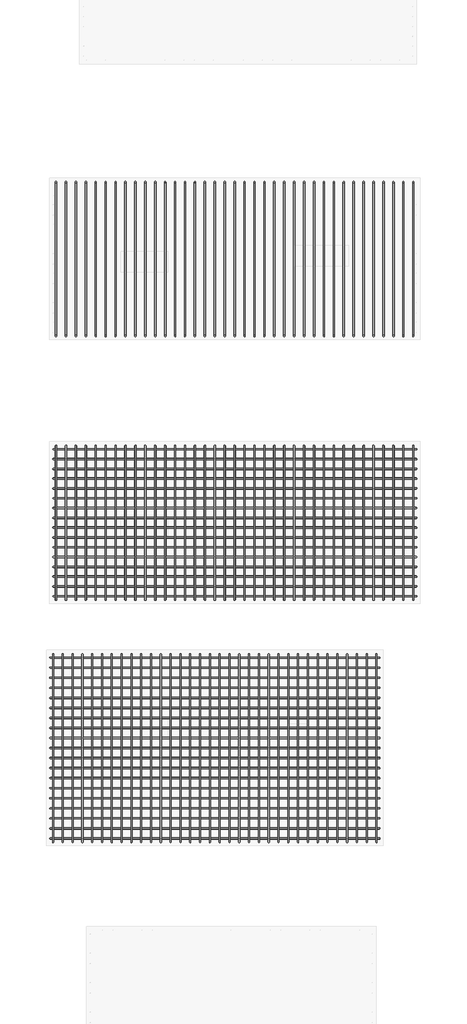
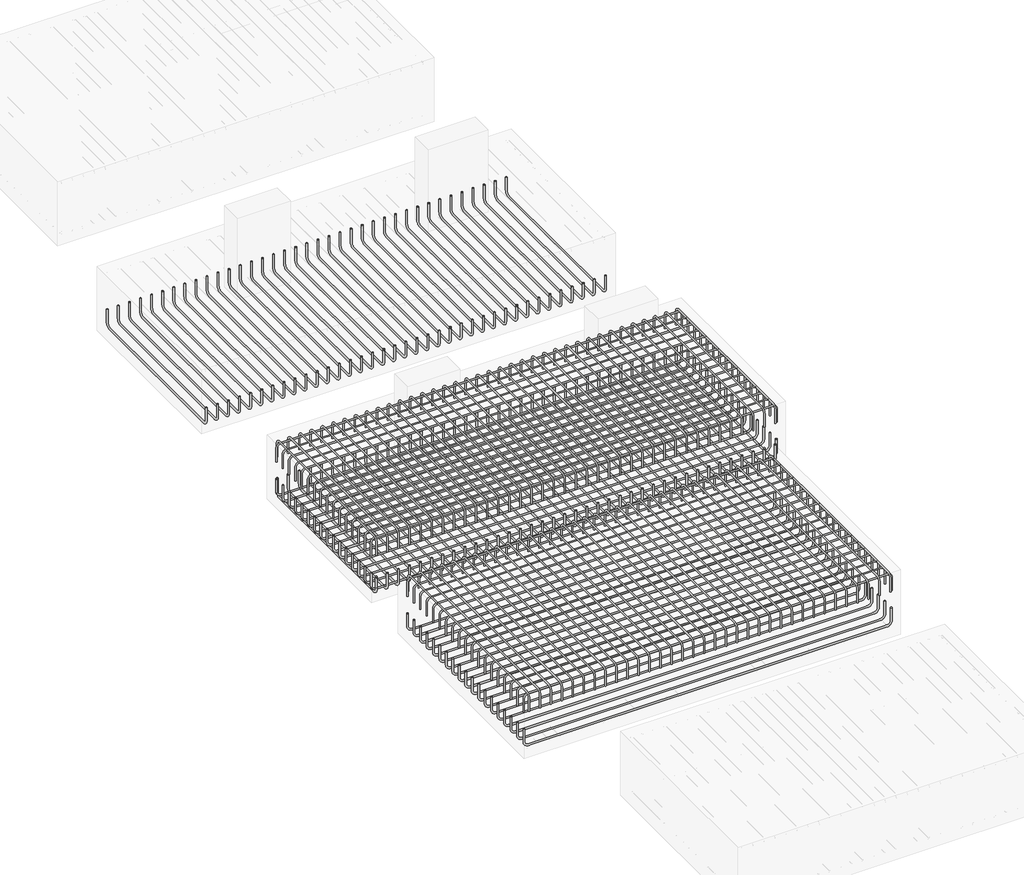
# One storey, part 7 of 21: 8 reinforcing bars.
"""IFC4 building model written with IfcOpenShell, lengths in millimetres."""

from ifc_helpers import new_model, si_unit, point, frame, origin, place, context, project, spatial, polyline, circle_curve, trimmed, segment, composite_curve, source, transform, mapped, element, save
from ifc_brep_helpers import swept_disk

model = new_model("IFC4")

# Units and contexts
model_context = context("Model", 3, world=origin())
ifc_project = project(units=[si_unit("LENGTHUNIT", "METRE", prefix="MILLI")], contexts=[model_context])

# Site, building, storey
site = spatial("IfcSite", under=ifc_project)
building = spatial("IfcBuilding", under=site)
storey = spatial("IfcBuildingStorey", under=building, Elevation=-1100.0)

# Reinforcing bars
placement = place(None, origin())
reinforcing_bar_shape = source(origin(), model_context, "Body", "SolidModel", [
    swept_disk(composite_curve([segment(polyline([(10485.4160849, 639.1704288, -1700.0), (10485.4160849, 639.1704288, -1882.5)]), True, "CONTINUOUS"), segment(trimmed(circle_curve(frame((10485.4160849, 581.6704288, -1882.5), z_axis=(-1.0, 0.0, 0.0), x_axis=(0.0, 57.5, 0.0)), 57.5), [point((10485.4160849, 639.1704288, -1882.5))], [point((10485.4160849, 581.6704288, -1940.0))], True, "CARTESIAN"), True, "CONTINUOUS"), segment(polyline([(10485.4160849, 581.6704288, -1940.0), (10485.4160849, -1583.3295712, -1940.0)]), True, "CONTINUOUS"), segment(trimmed(circle_curve(frame((10485.4160849, -1583.3295712, -1882.5), z_axis=(-1.0, 0.0, 0.0), x_axis=(0.0, 0.0, -57.5)), 57.5), [point((10485.4160849, -1583.3295712, -1940.0))], [point((10485.4160849, -1640.8295712, -1882.5))], True, "CARTESIAN"), True, "CONTINUOUS"), segment(polyline([(10485.4160849, -1640.8295712, -1882.5), (10485.4160849, -1640.8295712, -1700.0)]), True, "CONTINUOUS")], self_intersect=False), 10.0),
])
element("IfcReinforcingBar", 1, at=placement, inside=storey, context=model_context, shape_type="MappedRepresentation", body=[
    mapped(reinforcing_bar_shape, transform((0.0, 0.0, 0.0), x_axis=(1.0, 0.0, 0.0), y_axis=(0.0, 1.0, 0.0), z_axis=(0.0, 0.0, 1.0))),
    mapped(reinforcing_bar_shape, transform((147.2696553, 0.0, 0.0), x_axis=(1.0, 0.0, 0.0), y_axis=(0.0, 1.0, 0.0), z_axis=(0.0, 0.0, 1.0))),
    mapped(reinforcing_bar_shape, transform((294.5393106, 0.0, 0.0), x_axis=(1.0, 0.0, 0.0), y_axis=(0.0, 1.0, 0.0), z_axis=(0.0, 0.0, 1.0))),
    mapped(reinforcing_bar_shape, transform((441.8089659, 0.0, 0.0), x_axis=(1.0, 0.0, 0.0), y_axis=(0.0, 1.0, 0.0), z_axis=(0.0, 0.0, 1.0))),
    mapped(reinforcing_bar_shape, transform((589.0786213, 0.0, 0.0), x_axis=(1.0, 0.0, 0.0), y_axis=(0.0, 1.0, 0.0), z_axis=(0.0, 0.0, 1.0))),
    mapped(reinforcing_bar_shape, transform((736.3482766, 0.0, 0.0), x_axis=(1.0, 0.0, 0.0), y_axis=(0.0, 1.0, 0.0), z_axis=(0.0, 0.0, 1.0))),
    mapped(reinforcing_bar_shape, transform((883.6179319, 0.0, 0.0), x_axis=(1.0, 0.0, 0.0), y_axis=(0.0, 1.0, 0.0), z_axis=(0.0, 0.0, 1.0))),
    mapped(reinforcing_bar_shape, transform((1030.8875872, 0.0, 0.0), x_axis=(1.0, 0.0, 0.0), y_axis=(0.0, 1.0, 0.0), z_axis=(0.0, 0.0, 1.0))),
    mapped(reinforcing_bar_shape, transform((1178.1572425, 0.0, 0.0), x_axis=(1.0, 0.0, 0.0), y_axis=(0.0, 1.0, 0.0), z_axis=(0.0, 0.0, 1.0))),
    mapped(reinforcing_bar_shape, transform((1325.4268978, 0.0, 0.0), x_axis=(1.0, 0.0, 0.0), y_axis=(0.0, 1.0, 0.0), z_axis=(0.0, 0.0, 1.0))),
    mapped(reinforcing_bar_shape, transform((1472.6965532, 0.0, 0.0), x_axis=(1.0, 0.0, 0.0), y_axis=(0.0, 1.0, 0.0), z_axis=(0.0, 0.0, 1.0))),
    mapped(reinforcing_bar_shape, transform((1619.9662085, 0.0, 0.0), x_axis=(1.0, 0.0, 0.0), y_axis=(0.0, 1.0, 0.0), z_axis=(0.0, 0.0, 1.0))),
    mapped(reinforcing_bar_shape, transform((1767.2358638, 0.0, 0.0), x_axis=(1.0, 0.0, 0.0), y_axis=(0.0, 1.0, 0.0), z_axis=(0.0, 0.0, 1.0))),
    mapped(reinforcing_bar_shape, transform((1914.5055191, 0.0, 0.0), x_axis=(1.0, 0.0, 0.0), y_axis=(0.0, 1.0, 0.0), z_axis=(0.0, 0.0, 1.0))),
    mapped(reinforcing_bar_shape, transform((2061.7751744, 0.0, 0.0), x_axis=(1.0, 0.0, 0.0), y_axis=(0.0, 1.0, 0.0), z_axis=(0.0, 0.0, 1.0))),
    mapped(reinforcing_bar_shape, transform((2209.0448297, 0.0, 0.0), x_axis=(1.0, 0.0, 0.0), y_axis=(0.0, 1.0, 0.0), z_axis=(0.0, 0.0, 1.0))),
    mapped(reinforcing_bar_shape, transform((2356.314485, 0.0, 0.0), x_axis=(1.0, 0.0, 0.0), y_axis=(0.0, 1.0, 0.0), z_axis=(0.0, 0.0, 1.0))),
    mapped(reinforcing_bar_shape, transform((2503.5841404, 0.0, 0.0), x_axis=(1.0, 0.0, 0.0), y_axis=(0.0, 1.0, 0.0), z_axis=(0.0, 0.0, 1.0))),
    mapped(reinforcing_bar_shape, transform((2650.8537957, 0.0, 0.0), x_axis=(1.0, 0.0, 0.0), y_axis=(0.0, 1.0, 0.0), z_axis=(0.0, 0.0, 1.0))),
    mapped(reinforcing_bar_shape, transform((2798.123451, 0.0, 0.0), x_axis=(1.0, 0.0, 0.0), y_axis=(0.0, 1.0, 0.0), z_axis=(0.0, 0.0, 1.0))),
    mapped(reinforcing_bar_shape, transform((2945.3931063, 0.0, 0.0), x_axis=(1.0, 0.0, 0.0), y_axis=(0.0, 1.0, 0.0), z_axis=(0.0, 0.0, 1.0))),
    mapped(reinforcing_bar_shape, transform((3092.6627616, 0.0, 0.0), x_axis=(1.0, 0.0, 0.0), y_axis=(0.0, 1.0, 0.0), z_axis=(0.0, 0.0, 1.0))),
    mapped(reinforcing_bar_shape, transform((3239.9324169, 0.0, 0.0), x_axis=(1.0, 0.0, 0.0), y_axis=(0.0, 1.0, 0.0), z_axis=(0.0, 0.0, 1.0))),
    mapped(reinforcing_bar_shape, transform((3387.2020722, 0.0, 0.0), x_axis=(1.0, 0.0, 0.0), y_axis=(0.0, 1.0, 0.0), z_axis=(0.0, 0.0, 1.0))),
    mapped(reinforcing_bar_shape, transform((3534.4717276, 0.0, 0.0), x_axis=(1.0, 0.0, 0.0), y_axis=(0.0, 1.0, 0.0), z_axis=(0.0, 0.0, 1.0))),
    mapped(reinforcing_bar_shape, transform((3681.7413829, 0.0, 0.0), x_axis=(1.0, 0.0, 0.0), y_axis=(0.0, 1.0, 0.0), z_axis=(0.0, 0.0, 1.0))),
    mapped(reinforcing_bar_shape, transform((3829.0110382, 0.0, 0.0), x_axis=(1.0, 0.0, 0.0), y_axis=(0.0, 1.0, 0.0), z_axis=(0.0, 0.0, 1.0))),
    mapped(reinforcing_bar_shape, transform((3976.2806935, 0.0, 0.0), x_axis=(1.0, 0.0, 0.0), y_axis=(0.0, 1.0, 0.0), z_axis=(0.0, 0.0, 1.0))),
    mapped(reinforcing_bar_shape, transform((4123.5503488, 0.0, 0.0), x_axis=(1.0, 0.0, 0.0), y_axis=(0.0, 1.0, 0.0), z_axis=(0.0, 0.0, 1.0))),
    mapped(reinforcing_bar_shape, transform((4270.8200041, 0.0, 0.0), x_axis=(1.0, 0.0, 0.0), y_axis=(0.0, 1.0, 0.0), z_axis=(0.0, 0.0, 1.0))),
    mapped(reinforcing_bar_shape, transform((4418.0896595, 0.0, 0.0), x_axis=(1.0, 0.0, 0.0), y_axis=(0.0, 1.0, 0.0), z_axis=(0.0, 0.0, 1.0))),
    mapped(reinforcing_bar_shape, transform((4565.3593148, 0.0, 0.0), x_axis=(1.0, 0.0, 0.0), y_axis=(0.0, 1.0, 0.0), z_axis=(0.0, 0.0, 1.0))),
    mapped(reinforcing_bar_shape, transform((4712.6289701, 0.0, 0.0), x_axis=(1.0, 0.0, 0.0), y_axis=(0.0, 1.0, 0.0), z_axis=(0.0, 0.0, 1.0))),
    mapped(reinforcing_bar_shape, transform((4859.8986254, 0.0, 0.0), x_axis=(1.0, 0.0, 0.0), y_axis=(0.0, 1.0, 0.0), z_axis=(0.0, 0.0, 1.0))),
    mapped(reinforcing_bar_shape, transform((5007.1682807, 0.0, 0.0), x_axis=(1.0, 0.0, 0.0), y_axis=(0.0, 1.0, 0.0), z_axis=(0.0, 0.0, 1.0))),
    mapped(reinforcing_bar_shape, transform((5154.437936, 0.0, 0.0), x_axis=(1.0, 0.0, 0.0), y_axis=(0.0, 1.0, 0.0), z_axis=(0.0, 0.0, 1.0))),
    mapped(reinforcing_bar_shape, transform((5301.7075913, 0.0, 0.0), x_axis=(1.0, 0.0, 0.0), y_axis=(0.0, 1.0, 0.0), z_axis=(0.0, 0.0, 1.0))),
])
reinforcing_bar_2_shape = source(origin(), model_context, "Body", "SolidModel", [
    swept_disk(composite_curve([segment(polyline([(10485.4160849, -3270.8295712, -1700.0), (10485.4160849, -3270.8295712, -1882.5)]), True, "CONTINUOUS"), segment(trimmed(circle_curve(frame((10485.4160849, -3328.3295712, -1882.5), z_axis=(-1.0, 0.0, 0.0), x_axis=(0.0, 57.5, 0.0)), 57.5), [point((10485.4160849, -3270.8295712, -1882.5))], [point((10485.4160849, -3328.3295712, -1940.0))], True, "CARTESIAN"), True, "CONTINUOUS"), segment(polyline([(10485.4160849, -3328.3295712, -1940.0), (10485.4160849, -5493.3295712, -1940.0)]), True, "CONTINUOUS"), segment(trimmed(circle_curve(frame((10485.4160849, -5493.3295712, -1882.5), z_axis=(-1.0, 0.0, 0.0), x_axis=(0.0, 0.0, -57.5)), 57.5), [point((10485.4160849, -5493.3295712, -1940.0))], [point((10485.4160849, -5550.8295712, -1882.5))], True, "CARTESIAN"), True, "CONTINUOUS"), segment(polyline([(10485.4160849, -5550.8295712, -1882.5), (10485.4160849, -5550.8295712, -1700.0)]), True, "CONTINUOUS")], self_intersect=False), 10.0),
])
element("IfcReinforcingBar", 2, at=placement, inside=storey, context=model_context, shape_type="MappedRepresentation", body=[
    mapped(reinforcing_bar_2_shape, transform((0.0, 0.0, 0.0), x_axis=(1.0, 0.0, 0.0), y_axis=(0.0, 1.0, 0.0), z_axis=(0.0, 0.0, 1.0))),
    mapped(reinforcing_bar_2_shape, transform((147.2696553, 0.0, 0.0), x_axis=(1.0, 0.0, 0.0), y_axis=(0.0, 1.0, 0.0), z_axis=(0.0, 0.0, 1.0))),
    mapped(reinforcing_bar_2_shape, transform((294.5393106, 0.0, 0.0), x_axis=(1.0, 0.0, 0.0), y_axis=(0.0, 1.0, 0.0), z_axis=(0.0, 0.0, 1.0))),
    mapped(reinforcing_bar_2_shape, transform((441.8089659, 0.0, 0.0), x_axis=(1.0, 0.0, 0.0), y_axis=(0.0, 1.0, 0.0), z_axis=(0.0, 0.0, 1.0))),
    mapped(reinforcing_bar_2_shape, transform((589.0786213, 0.0, 0.0), x_axis=(1.0, 0.0, 0.0), y_axis=(0.0, 1.0, 0.0), z_axis=(0.0, 0.0, 1.0))),
    mapped(reinforcing_bar_2_shape, transform((736.3482766, 0.0, 0.0), x_axis=(1.0, 0.0, 0.0), y_axis=(0.0, 1.0, 0.0), z_axis=(0.0, 0.0, 1.0))),
    mapped(reinforcing_bar_2_shape, transform((883.6179319, 0.0, 0.0), x_axis=(1.0, 0.0, 0.0), y_axis=(0.0, 1.0, 0.0), z_axis=(0.0, 0.0, 1.0))),
    mapped(reinforcing_bar_2_shape, transform((1030.8875872, 0.0, 0.0), x_axis=(1.0, 0.0, 0.0), y_axis=(0.0, 1.0, 0.0), z_axis=(0.0, 0.0, 1.0))),
    mapped(reinforcing_bar_2_shape, transform((1178.1572425, 0.0, 0.0), x_axis=(1.0, 0.0, 0.0), y_axis=(0.0, 1.0, 0.0), z_axis=(0.0, 0.0, 1.0))),
    mapped(reinforcing_bar_2_shape, transform((1325.4268978, 0.0, 0.0), x_axis=(1.0, 0.0, 0.0), y_axis=(0.0, 1.0, 0.0), z_axis=(0.0, 0.0, 1.0))),
    mapped(reinforcing_bar_2_shape, transform((1472.6965532, 0.0, 0.0), x_axis=(1.0, 0.0, 0.0), y_axis=(0.0, 1.0, 0.0), z_axis=(0.0, 0.0, 1.0))),
    mapped(reinforcing_bar_2_shape, transform((1619.9662085, 0.0, 0.0), x_axis=(1.0, 0.0, 0.0), y_axis=(0.0, 1.0, 0.0), z_axis=(0.0, 0.0, 1.0))),
    mapped(reinforcing_bar_2_shape, transform((1767.2358638, 0.0, 0.0), x_axis=(1.0, 0.0, 0.0), y_axis=(0.0, 1.0, 0.0), z_axis=(0.0, 0.0, 1.0))),
    mapped(reinforcing_bar_2_shape, transform((1914.5055191, 0.0, 0.0), x_axis=(1.0, 0.0, 0.0), y_axis=(0.0, 1.0, 0.0), z_axis=(0.0, 0.0, 1.0))),
    mapped(reinforcing_bar_2_shape, transform((2061.7751744, 0.0, 0.0), x_axis=(1.0, 0.0, 0.0), y_axis=(0.0, 1.0, 0.0), z_axis=(0.0, 0.0, 1.0))),
    mapped(reinforcing_bar_2_shape, transform((2209.0448297, 0.0, 0.0), x_axis=(1.0, 0.0, 0.0), y_axis=(0.0, 1.0, 0.0), z_axis=(0.0, 0.0, 1.0))),
    mapped(reinforcing_bar_2_shape, transform((2356.314485, 0.0, 0.0), x_axis=(1.0, 0.0, 0.0), y_axis=(0.0, 1.0, 0.0), z_axis=(0.0, 0.0, 1.0))),
    mapped(reinforcing_bar_2_shape, transform((2503.5841404, 0.0, 0.0), x_axis=(1.0, 0.0, 0.0), y_axis=(0.0, 1.0, 0.0), z_axis=(0.0, 0.0, 1.0))),
    mapped(reinforcing_bar_2_shape, transform((2650.8537957, 0.0, 0.0), x_axis=(1.0, 0.0, 0.0), y_axis=(0.0, 1.0, 0.0), z_axis=(0.0, 0.0, 1.0))),
    mapped(reinforcing_bar_2_shape, transform((2798.123451, 0.0, 0.0), x_axis=(1.0, 0.0, 0.0), y_axis=(0.0, 1.0, 0.0), z_axis=(0.0, 0.0, 1.0))),
    mapped(reinforcing_bar_2_shape, transform((2945.3931063, 0.0, 0.0), x_axis=(1.0, 0.0, 0.0), y_axis=(0.0, 1.0, 0.0), z_axis=(0.0, 0.0, 1.0))),
    mapped(reinforcing_bar_2_shape, transform((3092.6627616, 0.0, 0.0), x_axis=(1.0, 0.0, 0.0), y_axis=(0.0, 1.0, 0.0), z_axis=(0.0, 0.0, 1.0))),
    mapped(reinforcing_bar_2_shape, transform((3239.9324169, 0.0, 0.0), x_axis=(1.0, 0.0, 0.0), y_axis=(0.0, 1.0, 0.0), z_axis=(0.0, 0.0, 1.0))),
    mapped(reinforcing_bar_2_shape, transform((3387.2020722, 0.0, 0.0), x_axis=(1.0, 0.0, 0.0), y_axis=(0.0, 1.0, 0.0), z_axis=(0.0, 0.0, 1.0))),
    mapped(reinforcing_bar_2_shape, transform((3534.4717276, 0.0, 0.0), x_axis=(1.0, 0.0, 0.0), y_axis=(0.0, 1.0, 0.0), z_axis=(0.0, 0.0, 1.0))),
    mapped(reinforcing_bar_2_shape, transform((3681.7413829, 0.0, 0.0), x_axis=(1.0, 0.0, 0.0), y_axis=(0.0, 1.0, 0.0), z_axis=(0.0, 0.0, 1.0))),
    mapped(reinforcing_bar_2_shape, transform((3829.0110382, 0.0, 0.0), x_axis=(1.0, 0.0, 0.0), y_axis=(0.0, 1.0, 0.0), z_axis=(0.0, 0.0, 1.0))),
    mapped(reinforcing_bar_2_shape, transform((3976.2806935, 0.0, 0.0), x_axis=(1.0, 0.0, 0.0), y_axis=(0.0, 1.0, 0.0), z_axis=(0.0, 0.0, 1.0))),
    mapped(reinforcing_bar_2_shape, transform((4123.5503488, 0.0, 0.0), x_axis=(1.0, 0.0, 0.0), y_axis=(0.0, 1.0, 0.0), z_axis=(0.0, 0.0, 1.0))),
    mapped(reinforcing_bar_2_shape, transform((4270.8200041, 0.0, 0.0), x_axis=(1.0, 0.0, 0.0), y_axis=(0.0, 1.0, 0.0), z_axis=(0.0, 0.0, 1.0))),
    mapped(reinforcing_bar_2_shape, transform((4418.0896595, 0.0, 0.0), x_axis=(1.0, 0.0, 0.0), y_axis=(0.0, 1.0, 0.0), z_axis=(0.0, 0.0, 1.0))),
    mapped(reinforcing_bar_2_shape, transform((4565.3593148, 0.0, 0.0), x_axis=(1.0, 0.0, 0.0), y_axis=(0.0, 1.0, 0.0), z_axis=(0.0, 0.0, 1.0))),
    mapped(reinforcing_bar_2_shape, transform((4712.6289701, 0.0, 0.0), x_axis=(1.0, 0.0, 0.0), y_axis=(0.0, 1.0, 0.0), z_axis=(0.0, 0.0, 1.0))),
    mapped(reinforcing_bar_2_shape, transform((4859.8986254, 0.0, 0.0), x_axis=(1.0, 0.0, 0.0), y_axis=(0.0, 1.0, 0.0), z_axis=(0.0, 0.0, 1.0))),
    mapped(reinforcing_bar_2_shape, transform((5007.1682807, 0.0, 0.0), x_axis=(1.0, 0.0, 0.0), y_axis=(0.0, 1.0, 0.0), z_axis=(0.0, 0.0, 1.0))),
    mapped(reinforcing_bar_2_shape, transform((5154.437936, 0.0, 0.0), x_axis=(1.0, 0.0, 0.0), y_axis=(0.0, 1.0, 0.0), z_axis=(0.0, 0.0, 1.0))),
    mapped(reinforcing_bar_2_shape, transform((5301.7075913, 0.0, 0.0), x_axis=(1.0, 0.0, 0.0), y_axis=(0.0, 1.0, 0.0), z_axis=(0.0, 0.0, 1.0))),
])
reinforcing_bar_3_shape = source(origin(), model_context, "Body", "SolidModel", [
    swept_disk(composite_curve([segment(polyline([(10485.4160849, -5552.8795712, -1400.0), (10485.4160849, -5552.8795712, -1213.4)]), True, "CONTINUOUS"), segment(trimmed(circle_curve(frame((10485.4160849, -5497.4295712, -1213.4), z_axis=(-1.0, 0.0, 0.0), x_axis=(0.0, -55.44999999999982, 0.0)), 55.45), [point((10485.4160849, -5552.8795712, -1213.4))], [point((10485.4160849, -5497.4295712, -1157.95))], True, "CARTESIAN"), True, "CONTINUOUS"), segment(polyline([(10485.4160849, -5497.4295712, -1157.95), (10485.4160849, -3324.2295712, -1157.95)]), True, "CONTINUOUS"), segment(trimmed(circle_curve(frame((10485.4160849, -3324.2295712, -1213.4), z_axis=(-1.0, 0.0, 0.0), x_axis=(0.0, 0.0, 55.450000000000045)), 55.45), [point((10485.4160849, -3324.2295712, -1157.95))], [point((10485.4160849, -3268.7795712, -1213.4))], True, "CARTESIAN"), True, "CONTINUOUS"), segment(polyline([(10485.4160849, -3268.7795712, -1213.4), (10485.4160849, -3268.7795712, -1400.0)]), True, "CONTINUOUS")], self_intersect=False), 7.95),
])
element("IfcReinforcingBar", 3, at=placement, inside=storey, context=model_context, shape_type="MappedRepresentation", body=[
    mapped(reinforcing_bar_3_shape, transform((0.0, 0.0, 0.0), x_axis=(1.0, 0.0, 0.0), y_axis=(0.0, 1.0, 0.0), z_axis=(0.0, 0.0, 1.0))),
    mapped(reinforcing_bar_3_shape, transform((147.2696553, 0.0, 0.0), x_axis=(1.0, 0.0, 0.0), y_axis=(0.0, 1.0, 0.0), z_axis=(0.0, 0.0, 1.0))),
    mapped(reinforcing_bar_3_shape, transform((294.5393106, 0.0, 0.0), x_axis=(1.0, 0.0, 0.0), y_axis=(0.0, 1.0, 0.0), z_axis=(0.0, 0.0, 1.0))),
    mapped(reinforcing_bar_3_shape, transform((441.8089659, 0.0, 0.0), x_axis=(1.0, 0.0, 0.0), y_axis=(0.0, 1.0, 0.0), z_axis=(0.0, 0.0, 1.0))),
    mapped(reinforcing_bar_3_shape, transform((589.0786213, 0.0, 0.0), x_axis=(1.0, 0.0, 0.0), y_axis=(0.0, 1.0, 0.0), z_axis=(0.0, 0.0, 1.0))),
    mapped(reinforcing_bar_3_shape, transform((736.3482766, 0.0, 0.0), x_axis=(1.0, 0.0, 0.0), y_axis=(0.0, 1.0, 0.0), z_axis=(0.0, 0.0, 1.0))),
    mapped(reinforcing_bar_3_shape, transform((883.6179319, 0.0, 0.0), x_axis=(1.0, 0.0, 0.0), y_axis=(0.0, 1.0, 0.0), z_axis=(0.0, 0.0, 1.0))),
    mapped(reinforcing_bar_3_shape, transform((1030.8875872, 0.0, 0.0), x_axis=(1.0, 0.0, 0.0), y_axis=(0.0, 1.0, 0.0), z_axis=(0.0, 0.0, 1.0))),
    mapped(reinforcing_bar_3_shape, transform((1178.1572425, 0.0, 0.0), x_axis=(1.0, 0.0, 0.0), y_axis=(0.0, 1.0, 0.0), z_axis=(0.0, 0.0, 1.0))),
    mapped(reinforcing_bar_3_shape, transform((1325.4268978, 0.0, 0.0), x_axis=(1.0, 0.0, 0.0), y_axis=(0.0, 1.0, 0.0), z_axis=(0.0, 0.0, 1.0))),
    mapped(reinforcing_bar_3_shape, transform((1472.6965532, 0.0, 0.0), x_axis=(1.0, 0.0, 0.0), y_axis=(0.0, 1.0, 0.0), z_axis=(0.0, 0.0, 1.0))),
    mapped(reinforcing_bar_3_shape, transform((1619.9662085, 0.0, 0.0), x_axis=(1.0, 0.0, 0.0), y_axis=(0.0, 1.0, 0.0), z_axis=(0.0, 0.0, 1.0))),
    mapped(reinforcing_bar_3_shape, transform((1767.2358638, 0.0, 0.0), x_axis=(1.0, 0.0, 0.0), y_axis=(0.0, 1.0, 0.0), z_axis=(0.0, 0.0, 1.0))),
    mapped(reinforcing_bar_3_shape, transform((1914.5055191, 0.0, 0.0), x_axis=(1.0, 0.0, 0.0), y_axis=(0.0, 1.0, 0.0), z_axis=(0.0, 0.0, 1.0))),
    mapped(reinforcing_bar_3_shape, transform((2061.7751744, 0.0, 0.0), x_axis=(1.0, 0.0, 0.0), y_axis=(0.0, 1.0, 0.0), z_axis=(0.0, 0.0, 1.0))),
    mapped(reinforcing_bar_3_shape, transform((2209.0448297, 0.0, 0.0), x_axis=(1.0, 0.0, 0.0), y_axis=(0.0, 1.0, 0.0), z_axis=(0.0, 0.0, 1.0))),
    mapped(reinforcing_bar_3_shape, transform((2356.314485, 0.0, 0.0), x_axis=(1.0, 0.0, 0.0), y_axis=(0.0, 1.0, 0.0), z_axis=(0.0, 0.0, 1.0))),
    mapped(reinforcing_bar_3_shape, transform((2503.5841404, 0.0, 0.0), x_axis=(1.0, 0.0, 0.0), y_axis=(0.0, 1.0, 0.0), z_axis=(0.0, 0.0, 1.0))),
    mapped(reinforcing_bar_3_shape, transform((2650.8537957, 0.0, 0.0), x_axis=(1.0, 0.0, 0.0), y_axis=(0.0, 1.0, 0.0), z_axis=(0.0, 0.0, 1.0))),
    mapped(reinforcing_bar_3_shape, transform((2798.123451, 0.0, 0.0), x_axis=(1.0, 0.0, 0.0), y_axis=(0.0, 1.0, 0.0), z_axis=(0.0, 0.0, 1.0))),
    mapped(reinforcing_bar_3_shape, transform((2945.3931063, 0.0, 0.0), x_axis=(1.0, 0.0, 0.0), y_axis=(0.0, 1.0, 0.0), z_axis=(0.0, 0.0, 1.0))),
    mapped(reinforcing_bar_3_shape, transform((3092.6627616, 0.0, 0.0), x_axis=(1.0, 0.0, 0.0), y_axis=(0.0, 1.0, 0.0), z_axis=(0.0, 0.0, 1.0))),
    mapped(reinforcing_bar_3_shape, transform((3239.9324169, 0.0, 0.0), x_axis=(1.0, 0.0, 0.0), y_axis=(0.0, 1.0, 0.0), z_axis=(0.0, 0.0, 1.0))),
    mapped(reinforcing_bar_3_shape, transform((3387.2020722, 0.0, 0.0), x_axis=(1.0, 0.0, 0.0), y_axis=(0.0, 1.0, 0.0), z_axis=(0.0, 0.0, 1.0))),
    mapped(reinforcing_bar_3_shape, transform((3534.4717276, 0.0, 0.0), x_axis=(1.0, 0.0, 0.0), y_axis=(0.0, 1.0, 0.0), z_axis=(0.0, 0.0, 1.0))),
    mapped(reinforcing_bar_3_shape, transform((3681.7413829, 0.0, 0.0), x_axis=(1.0, 0.0, 0.0), y_axis=(0.0, 1.0, 0.0), z_axis=(0.0, 0.0, 1.0))),
    mapped(reinforcing_bar_3_shape, transform((3829.0110382, 0.0, 0.0), x_axis=(1.0, 0.0, 0.0), y_axis=(0.0, 1.0, 0.0), z_axis=(0.0, 0.0, 1.0))),
    mapped(reinforcing_bar_3_shape, transform((3976.2806935, 0.0, 0.0), x_axis=(1.0, 0.0, 0.0), y_axis=(0.0, 1.0, 0.0), z_axis=(0.0, 0.0, 1.0))),
    mapped(reinforcing_bar_3_shape, transform((4123.5503488, 0.0, 0.0), x_axis=(1.0, 0.0, 0.0), y_axis=(0.0, 1.0, 0.0), z_axis=(0.0, 0.0, 1.0))),
    mapped(reinforcing_bar_3_shape, transform((4270.8200041, 0.0, 0.0), x_axis=(1.0, 0.0, 0.0), y_axis=(0.0, 1.0, 0.0), z_axis=(0.0, 0.0, 1.0))),
    mapped(reinforcing_bar_3_shape, transform((4418.0896595, 0.0, 0.0), x_axis=(1.0, 0.0, 0.0), y_axis=(0.0, 1.0, 0.0), z_axis=(0.0, 0.0, 1.0))),
    mapped(reinforcing_bar_3_shape, transform((4565.3593148, 0.0, 0.0), x_axis=(1.0, 0.0, 0.0), y_axis=(0.0, 1.0, 0.0), z_axis=(0.0, 0.0, 1.0))),
    mapped(reinforcing_bar_3_shape, transform((4712.6289701, 0.0, 0.0), x_axis=(1.0, 0.0, 0.0), y_axis=(0.0, 1.0, 0.0), z_axis=(0.0, 0.0, 1.0))),
    mapped(reinforcing_bar_3_shape, transform((4859.8986254, 0.0, 0.0), x_axis=(1.0, 0.0, 0.0), y_axis=(0.0, 1.0, 0.0), z_axis=(0.0, 0.0, 1.0))),
    mapped(reinforcing_bar_3_shape, transform((5007.1682807, 0.0, 0.0), x_axis=(1.0, 0.0, 0.0), y_axis=(0.0, 1.0, 0.0), z_axis=(0.0, 0.0, 1.0))),
    mapped(reinforcing_bar_3_shape, transform((5154.437936, 0.0, 0.0), x_axis=(1.0, 0.0, 0.0), y_axis=(0.0, 1.0, 0.0), z_axis=(0.0, 0.0, 1.0))),
    mapped(reinforcing_bar_3_shape, transform((5301.7075913, 0.0, 0.0), x_axis=(1.0, 0.0, 0.0), y_axis=(0.0, 1.0, 0.0), z_axis=(0.0, 0.0, 1.0))),
])
reinforcing_bar_4_shape = source(origin(), model_context, "Body", "SolidModel", [
    swept_disk(composite_curve([segment(polyline([(10447.1173137, -3320.6137352, -1428.1111113), (10447.1173137, -3320.6137352, -1241.5111113)]), True, "CONTINUOUS"), segment(trimmed(circle_curve(frame((10502.5673137, -3320.6137352, -1241.5111113), z_axis=(0.0, 1.0, 0.0), x_axis=(-55.44999999999891, 0.0, 0.0)), 55.45), [point((10447.1173137, -3320.6137352, -1241.5111113))], [point((10502.5673137, -3320.6137352, -1186.0611113))], True, "CARTESIAN"), True, "CONTINUOUS"), segment(polyline([(10502.5673137, -3320.6137352, -1186.0611113), (15775.7673137, -3320.6137352, -1186.0611113)]), True, "CONTINUOUS"), segment(trimmed(circle_curve(frame((15775.7673137, -3320.6137352, -1241.5111113), z_axis=(0.0, 1.0, 0.0), x_axis=(0.0, 0.0, 55.450000000000045)), 55.45), [point((15775.7673137, -3320.6137352, -1186.0611113))], [point((15831.2173137, -3320.6137352, -1241.5111113))], True, "CARTESIAN"), True, "CONTINUOUS"), segment(polyline([(15831.2173137, -3320.6137352, -1241.5111113), (15831.2173137, -3320.6137352, -1428.1111113)]), True, "CONTINUOUS")], self_intersect=False), 7.95),
])
element("IfcReinforcingBar", 4, at=placement, inside=storey, context=model_context, shape_type="MappedRepresentation", body=[
    mapped(reinforcing_bar_4_shape, transform((0.0, 0.0, 0.0), x_axis=(1.0, 0.0, 0.0), y_axis=(0.0, 1.0, 0.0), z_axis=(0.0, 0.0, 1.0))),
    mapped(reinforcing_bar_4_shape, transform((0.0, -145.2528929, 0.0), x_axis=(1.0, 0.0, 0.0), y_axis=(0.0, 1.0, 0.0), z_axis=(0.0, 0.0, 1.0))),
    mapped(reinforcing_bar_4_shape, transform((0.0, -290.5057858, 0.0), x_axis=(1.0, 0.0, 0.0), y_axis=(0.0, 1.0, 0.0), z_axis=(0.0, 0.0, 1.0))),
    mapped(reinforcing_bar_4_shape, transform((0.0, -435.7586787, 0.0), x_axis=(1.0, 0.0, 0.0), y_axis=(0.0, 1.0, 0.0), z_axis=(0.0, 0.0, 1.0))),
    mapped(reinforcing_bar_4_shape, transform((0.0, -581.0115716, 0.0), x_axis=(1.0, 0.0, 0.0), y_axis=(0.0, 1.0, 0.0), z_axis=(0.0, 0.0, 1.0))),
    mapped(reinforcing_bar_4_shape, transform((0.0, -726.2644645, 0.0), x_axis=(1.0, 0.0, 0.0), y_axis=(0.0, 1.0, 0.0), z_axis=(0.0, 0.0, 1.0))),
    mapped(reinforcing_bar_4_shape, transform((0.0, -871.5173574, 0.0), x_axis=(1.0, 0.0, 0.0), y_axis=(0.0, 1.0, 0.0), z_axis=(0.0, 0.0, 1.0))),
    mapped(reinforcing_bar_4_shape, transform((0.0, -1016.7702503, 0.0), x_axis=(1.0, 0.0, 0.0), y_axis=(0.0, 1.0, 0.0), z_axis=(0.0, 0.0, 1.0))),
    mapped(reinforcing_bar_4_shape, transform((0.0, -1162.0231432, 0.0), x_axis=(1.0, 0.0, 0.0), y_axis=(0.0, 1.0, 0.0), z_axis=(0.0, 0.0, 1.0))),
    mapped(reinforcing_bar_4_shape, transform((0.0, -1307.276036, 0.0), x_axis=(1.0, 0.0, 0.0), y_axis=(0.0, 1.0, 0.0), z_axis=(0.0, 0.0, 1.0))),
    mapped(reinforcing_bar_4_shape, transform((0.0, -1452.5289289, 0.0), x_axis=(1.0, 0.0, 0.0), y_axis=(0.0, 1.0, 0.0), z_axis=(0.0, 0.0, 1.0))),
    mapped(reinforcing_bar_4_shape, transform((0.0, -1597.7818218, 0.0), x_axis=(1.0, 0.0, 0.0), y_axis=(0.0, 1.0, 0.0), z_axis=(0.0, 0.0, 1.0))),
    mapped(reinforcing_bar_4_shape, transform((0.0, -1743.0347147, 0.0), x_axis=(1.0, 0.0, 0.0), y_axis=(0.0, 1.0, 0.0), z_axis=(0.0, 0.0, 1.0))),
    mapped(reinforcing_bar_4_shape, transform((0.0, -1888.2876076, 0.0), x_axis=(1.0, 0.0, 0.0), y_axis=(0.0, 1.0, 0.0), z_axis=(0.0, 0.0, 1.0))),
    mapped(reinforcing_bar_4_shape, transform((0.0, -2033.5405005, 0.0), x_axis=(1.0, 0.0, 0.0), y_axis=(0.0, 1.0, 0.0), z_axis=(0.0, 0.0, 1.0))),
    mapped(reinforcing_bar_4_shape, transform((0.0, -2178.7933934, 0.0), x_axis=(1.0, 0.0, 0.0), y_axis=(0.0, 1.0, 0.0), z_axis=(0.0, 0.0, 1.0))),
])
reinforcing_bar_5_shape = source(origin(), model_context, "Body", "SolidModel", [
    swept_disk(composite_curve([segment(polyline([(10449.1673137, -5499.4071286, -1669.8442859), (10449.1673137, -5499.4071286, -1852.3442859)]), True, "CONTINUOUS"), segment(trimmed(circle_curve(frame((10506.6673137, -5499.4071286, -1852.3442859), z_axis=(0.0, -1.0, 0.0), x_axis=(-57.5, 0.0, 0.0)), 57.5), [point((10449.1673137, -5499.4071286, -1852.3442859))], [point((10506.6673137, -5499.4071286, -1909.8442859))], True, "CARTESIAN"), True, "CONTINUOUS"), segment(polyline([(10506.6673137, -5499.4071286, -1909.8442859), (15771.6673137, -5499.4071286, -1909.8442859)]), True, "CONTINUOUS"), segment(trimmed(circle_curve(frame((15771.6673137, -5499.4071286, -1852.3442859), z_axis=(0.0, -1.0, 0.0), x_axis=(0.0, 0.0, -57.5)), 57.5), [point((15771.6673137, -5499.4071286, -1909.8442859))], [point((15829.1673137, -5499.4071286, -1852.3442859))], True, "CARTESIAN"), True, "CONTINUOUS"), segment(polyline([(15829.1673137, -5499.4071286, -1852.3442859), (15829.1673137, -5499.4071286, -1669.8442859)]), True, "CONTINUOUS")], self_intersect=False), 10.0),
])
element("IfcReinforcingBar", 5, at=placement, inside=storey, context=model_context, shape_type="MappedRepresentation", body=[
    mapped(reinforcing_bar_5_shape, transform((0.0, 0.0, 0.0), x_axis=(1.0, 0.0, 0.0), y_axis=(0.0, 1.0, 0.0), z_axis=(0.0, 0.0, 1.0))),
    mapped(reinforcing_bar_5_shape, transform((0.0, 145.2528929, 0.0), x_axis=(1.0, 0.0, 0.0), y_axis=(0.0, 1.0, 0.0), z_axis=(0.0, 0.0, 1.0))),
    mapped(reinforcing_bar_5_shape, transform((0.0, 290.5057858, 0.0), x_axis=(1.0, 0.0, 0.0), y_axis=(0.0, 1.0, 0.0), z_axis=(0.0, 0.0, 1.0))),
    mapped(reinforcing_bar_5_shape, transform((0.0, 435.7586787, 0.0), x_axis=(1.0, 0.0, 0.0), y_axis=(0.0, 1.0, 0.0), z_axis=(0.0, 0.0, 1.0))),
    mapped(reinforcing_bar_5_shape, transform((0.0, 581.0115716, 0.0), x_axis=(1.0, 0.0, 0.0), y_axis=(0.0, 1.0, 0.0), z_axis=(0.0, 0.0, 1.0))),
    mapped(reinforcing_bar_5_shape, transform((0.0, 726.2644645, 0.0), x_axis=(1.0, 0.0, 0.0), y_axis=(0.0, 1.0, 0.0), z_axis=(0.0, 0.0, 1.0))),
    mapped(reinforcing_bar_5_shape, transform((0.0, 871.5173574, 0.0), x_axis=(1.0, 0.0, 0.0), y_axis=(0.0, 1.0, 0.0), z_axis=(0.0, 0.0, 1.0))),
    mapped(reinforcing_bar_5_shape, transform((0.0, 1016.7702503, 0.0), x_axis=(1.0, 0.0, 0.0), y_axis=(0.0, 1.0, 0.0), z_axis=(0.0, 0.0, 1.0))),
    mapped(reinforcing_bar_5_shape, transform((0.0, 1162.0231432, 0.0), x_axis=(1.0, 0.0, 0.0), y_axis=(0.0, 1.0, 0.0), z_axis=(0.0, 0.0, 1.0))),
    mapped(reinforcing_bar_5_shape, transform((0.0, 1307.276036, 0.0), x_axis=(1.0, 0.0, 0.0), y_axis=(0.0, 1.0, 0.0), z_axis=(0.0, 0.0, 1.0))),
    mapped(reinforcing_bar_5_shape, transform((0.0, 1452.5289289, 0.0), x_axis=(1.0, 0.0, 0.0), y_axis=(0.0, 1.0, 0.0), z_axis=(0.0, 0.0, 1.0))),
    mapped(reinforcing_bar_5_shape, transform((0.0, 1597.7818218, 0.0), x_axis=(1.0, 0.0, 0.0), y_axis=(0.0, 1.0, 0.0), z_axis=(0.0, 0.0, 1.0))),
    mapped(reinforcing_bar_5_shape, transform((0.0, 1743.0347147, 0.0), x_axis=(1.0, 0.0, 0.0), y_axis=(0.0, 1.0, 0.0), z_axis=(0.0, 0.0, 1.0))),
    mapped(reinforcing_bar_5_shape, transform((0.0, 1888.2876076, 0.0), x_axis=(1.0, 0.0, 0.0), y_axis=(0.0, 1.0, 0.0), z_axis=(0.0, 0.0, 1.0))),
    mapped(reinforcing_bar_5_shape, transform((0.0, 2033.5405005, 0.0), x_axis=(1.0, 0.0, 0.0), y_axis=(0.0, 1.0, 0.0), z_axis=(0.0, 0.0, 1.0))),
    mapped(reinforcing_bar_5_shape, transform((0.0, 2178.7933934, 0.0), x_axis=(1.0, 0.0, 0.0), y_axis=(0.0, 1.0, 0.0), z_axis=(0.0, 0.0, 1.0))),
])
reinforcing_bar_6_shape = source(origin(), model_context, "Body", "SolidModel", [
    swept_disk(composite_curve([segment(polyline([(10440.4160849, -9142.8795712, -1400.0), (10440.4160849, -9142.8795712, -1213.4)]), True, "CONTINUOUS"), segment(trimmed(circle_curve(frame((10440.4160849, -9087.4295712, -1213.4), z_axis=(-1.0, 0.0, 0.0), x_axis=(0.0, -55.44999999999891, 0.0)), 55.45), [point((10440.4160849, -9142.8795712, -1213.4))], [point((10440.4160849, -9087.4295712, -1157.95))], True, "CARTESIAN"), True, "CONTINUOUS"), segment(polyline([(10440.4160849, -9087.4295712, -1157.95), (10440.4160849, -6414.2295712, -1157.95)]), True, "CONTINUOUS"), segment(trimmed(circle_curve(frame((10440.4160849, -6414.2295712, -1213.4), z_axis=(-1.0, 0.0, 0.0), x_axis=(0.0, 0.0, 55.450000000000045)), 55.45), [point((10440.4160849, -6414.2295712, -1157.95))], [point((10440.4160849, -6358.7795712, -1213.4))], True, "CARTESIAN"), True, "CONTINUOUS"), segment(polyline([(10440.4160849, -6358.7795712, -1213.4), (10440.4160849, -6358.7795712, -1400.0)]), True, "CONTINUOUS")], self_intersect=False), 7.95),
])
element("IfcReinforcingBar", 6, at=placement, inside=storey, context=model_context, shape_type="MappedRepresentation", body=[
    mapped(reinforcing_bar_6_shape, transform((0.0, 0.0, 0.0), x_axis=(1.0, 0.0, 0.0), y_axis=(0.0, 1.0, 0.0), z_axis=(0.0, 0.0, 1.0))),
    mapped(reinforcing_bar_6_shape, transform((145.5062906, 0.0, 0.0), x_axis=(1.0, 0.0, 0.0), y_axis=(0.0, 1.0, 0.0), z_axis=(0.0, 0.0, 1.0))),
    mapped(reinforcing_bar_6_shape, transform((291.0125813, 0.0, 0.0), x_axis=(1.0, 0.0, 0.0), y_axis=(0.0, 1.0, 0.0), z_axis=(0.0, 0.0, 1.0))),
    mapped(reinforcing_bar_6_shape, transform((436.5188719, 0.0, 0.0), x_axis=(1.0, 0.0, 0.0), y_axis=(0.0, 1.0, 0.0), z_axis=(0.0, 0.0, 1.0))),
    mapped(reinforcing_bar_6_shape, transform((582.0251626, 0.0, 0.0), x_axis=(1.0, 0.0, 0.0), y_axis=(0.0, 1.0, 0.0), z_axis=(0.0, 0.0, 1.0))),
    mapped(reinforcing_bar_6_shape, transform((727.5314532, 0.0, 0.0), x_axis=(1.0, 0.0, 0.0), y_axis=(0.0, 1.0, 0.0), z_axis=(0.0, 0.0, 1.0))),
    mapped(reinforcing_bar_6_shape, transform((873.0377439, 0.0, 0.0), x_axis=(1.0, 0.0, 0.0), y_axis=(0.0, 1.0, 0.0), z_axis=(0.0, 0.0, 1.0))),
    mapped(reinforcing_bar_6_shape, transform((1018.5440345, 0.0, 0.0), x_axis=(1.0, 0.0, 0.0), y_axis=(0.0, 1.0, 0.0), z_axis=(0.0, 0.0, 1.0))),
    mapped(reinforcing_bar_6_shape, transform((1164.0503252, 0.0, 0.0), x_axis=(1.0, 0.0, 0.0), y_axis=(0.0, 1.0, 0.0), z_axis=(0.0, 0.0, 1.0))),
    mapped(reinforcing_bar_6_shape, transform((1309.5566158, 0.0, 0.0), x_axis=(1.0, 0.0, 0.0), y_axis=(0.0, 1.0, 0.0), z_axis=(0.0, 0.0, 1.0))),
    mapped(reinforcing_bar_6_shape, transform((1455.0629065, 0.0, 0.0), x_axis=(1.0, 0.0, 0.0), y_axis=(0.0, 1.0, 0.0), z_axis=(0.0, 0.0, 1.0))),
    mapped(reinforcing_bar_6_shape, transform((1600.5691971, 0.0, 0.0), x_axis=(1.0, 0.0, 0.0), y_axis=(0.0, 1.0, 0.0), z_axis=(0.0, 0.0, 1.0))),
    mapped(reinforcing_bar_6_shape, transform((1746.0754878, 0.0, 0.0), x_axis=(1.0, 0.0, 0.0), y_axis=(0.0, 1.0, 0.0), z_axis=(0.0, 0.0, 1.0))),
    mapped(reinforcing_bar_6_shape, transform((1891.5817784, 0.0, 0.0), x_axis=(1.0, 0.0, 0.0), y_axis=(0.0, 1.0, 0.0), z_axis=(0.0, 0.0, 1.0))),
    mapped(reinforcing_bar_6_shape, transform((2037.0880691, 0.0, 0.0), x_axis=(1.0, 0.0, 0.0), y_axis=(0.0, 1.0, 0.0), z_axis=(0.0, 0.0, 1.0))),
    mapped(reinforcing_bar_6_shape, transform((2182.5943597, 0.0, 0.0), x_axis=(1.0, 0.0, 0.0), y_axis=(0.0, 1.0, 0.0), z_axis=(0.0, 0.0, 1.0))),
    mapped(reinforcing_bar_6_shape, transform((2328.1006504, 0.0, 0.0), x_axis=(1.0, 0.0, 0.0), y_axis=(0.0, 1.0, 0.0), z_axis=(0.0, 0.0, 1.0))),
    mapped(reinforcing_bar_6_shape, transform((2473.606941, 0.0, 0.0), x_axis=(1.0, 0.0, 0.0), y_axis=(0.0, 1.0, 0.0), z_axis=(0.0, 0.0, 1.0))),
    mapped(reinforcing_bar_6_shape, transform((2619.1132316, 0.0, 0.0), x_axis=(1.0, 0.0, 0.0), y_axis=(0.0, 1.0, 0.0), z_axis=(0.0, 0.0, 1.0))),
    mapped(reinforcing_bar_6_shape, transform((2764.6195223, 0.0, 0.0), x_axis=(1.0, 0.0, 0.0), y_axis=(0.0, 1.0, 0.0), z_axis=(0.0, 0.0, 1.0))),
    mapped(reinforcing_bar_6_shape, transform((2910.1258129, 0.0, 0.0), x_axis=(1.0, 0.0, 0.0), y_axis=(0.0, 1.0, 0.0), z_axis=(0.0, 0.0, 1.0))),
    mapped(reinforcing_bar_6_shape, transform((3055.6321036, 0.0, 0.0), x_axis=(1.0, 0.0, 0.0), y_axis=(0.0, 1.0, 0.0), z_axis=(0.0, 0.0, 1.0))),
    mapped(reinforcing_bar_6_shape, transform((3201.1383942, 0.0, 0.0), x_axis=(1.0, 0.0, 0.0), y_axis=(0.0, 1.0, 0.0), z_axis=(0.0, 0.0, 1.0))),
    mapped(reinforcing_bar_6_shape, transform((3346.6446849, 0.0, 0.0), x_axis=(1.0, 0.0, 0.0), y_axis=(0.0, 1.0, 0.0), z_axis=(0.0, 0.0, 1.0))),
    mapped(reinforcing_bar_6_shape, transform((3492.1509755, 0.0, 0.0), x_axis=(1.0, 0.0, 0.0), y_axis=(0.0, 1.0, 0.0), z_axis=(0.0, 0.0, 1.0))),
    mapped(reinforcing_bar_6_shape, transform((3637.6572662, 0.0, 0.0), x_axis=(1.0, 0.0, 0.0), y_axis=(0.0, 1.0, 0.0), z_axis=(0.0, 0.0, 1.0))),
    mapped(reinforcing_bar_6_shape, transform((3783.1635568, 0.0, 0.0), x_axis=(1.0, 0.0, 0.0), y_axis=(0.0, 1.0, 0.0), z_axis=(0.0, 0.0, 1.0))),
    mapped(reinforcing_bar_6_shape, transform((3928.6698475, 0.0, 0.0), x_axis=(1.0, 0.0, 0.0), y_axis=(0.0, 1.0, 0.0), z_axis=(0.0, 0.0, 1.0))),
    mapped(reinforcing_bar_6_shape, transform((4074.1761381, 0.0, 0.0), x_axis=(1.0, 0.0, 0.0), y_axis=(0.0, 1.0, 0.0), z_axis=(0.0, 0.0, 1.0))),
    mapped(reinforcing_bar_6_shape, transform((4219.6824288, 0.0, 0.0), x_axis=(1.0, 0.0, 0.0), y_axis=(0.0, 1.0, 0.0), z_axis=(0.0, 0.0, 1.0))),
    mapped(reinforcing_bar_6_shape, transform((4365.1887194, 0.0, 0.0), x_axis=(1.0, 0.0, 0.0), y_axis=(0.0, 1.0, 0.0), z_axis=(0.0, 0.0, 1.0))),
    mapped(reinforcing_bar_6_shape, transform((4510.6950101, 0.0, 0.0), x_axis=(1.0, 0.0, 0.0), y_axis=(0.0, 1.0, 0.0), z_axis=(0.0, 0.0, 1.0))),
    mapped(reinforcing_bar_6_shape, transform((4656.2013007, 0.0, 0.0), x_axis=(1.0, 0.0, 0.0), y_axis=(0.0, 1.0, 0.0), z_axis=(0.0, 0.0, 1.0))),
    mapped(reinforcing_bar_6_shape, transform((4801.7075913, 0.0, 0.0), x_axis=(1.0, 0.0, 0.0), y_axis=(0.0, 1.0, 0.0), z_axis=(0.0, 0.0, 1.0))),
])
reinforcing_bar_7_shape = source(origin(), model_context, "Body", "SolidModel", [
    swept_disk(composite_curve([segment(polyline([(10402.1173137, -6410.6137352, -1428.1111113), (10402.1173137, -6410.6137352, -1241.5111113)]), True, "CONTINUOUS"), segment(trimmed(circle_curve(frame((10457.5673137, -6410.6137352, -1241.5111113), z_axis=(0.0, 1.0, 0.0), x_axis=(-55.44999999999891, 0.0, 0.0)), 55.45), [point((10402.1173137, -6410.6137352, -1241.5111113))], [point((10457.5673137, -6410.6137352, -1186.0611113))], True, "CARTESIAN"), True, "CONTINUOUS"), segment(polyline([(10457.5673137, -6410.6137352, -1186.0611113), (15230.7673137, -6410.6137352, -1186.0611113)]), True, "CONTINUOUS"), segment(trimmed(circle_curve(frame((15230.7673137, -6410.6137352, -1241.5111113), z_axis=(0.0, 1.0, 0.0), x_axis=(0.0, 0.0, 55.450000000000045)), 55.45), [point((15230.7673137, -6410.6137352, -1186.0611113))], [point((15286.2173137, -6410.6137352, -1241.5111113))], True, "CARTESIAN"), True, "CONTINUOUS"), segment(polyline([(15286.2173137, -6410.6137352, -1241.5111113), (15286.2173137, -6410.6137352, -1428.1111113)]), True, "CONTINUOUS")], self_intersect=False), 7.95),
])
element("IfcReinforcingBar", 7, at=placement, inside=storey, context=model_context, shape_type="MappedRepresentation", body=[
    mapped(reinforcing_bar_7_shape, transform((0.0, 0.0, 0.0), x_axis=(1.0, 0.0, 0.0), y_axis=(0.0, 1.0, 0.0), z_axis=(0.0, 0.0, 1.0))),
    mapped(reinforcing_bar_7_shape, transform((0.0, -148.8218552, 0.0), x_axis=(1.0, 0.0, 0.0), y_axis=(0.0, 1.0, 0.0), z_axis=(0.0, 0.0, 1.0))),
    mapped(reinforcing_bar_7_shape, transform((0.0, -297.6437104, 0.0), x_axis=(1.0, 0.0, 0.0), y_axis=(0.0, 1.0, 0.0), z_axis=(0.0, 0.0, 1.0))),
    mapped(reinforcing_bar_7_shape, transform((0.0, -446.4655656, 0.0), x_axis=(1.0, 0.0, 0.0), y_axis=(0.0, 1.0, 0.0), z_axis=(0.0, 0.0, 1.0))),
    mapped(reinforcing_bar_7_shape, transform((0.0, -595.2874208, 0.0), x_axis=(1.0, 0.0, 0.0), y_axis=(0.0, 1.0, 0.0), z_axis=(0.0, 0.0, 1.0))),
    mapped(reinforcing_bar_7_shape, transform((0.0, -744.1092759, 0.0), x_axis=(1.0, 0.0, 0.0), y_axis=(0.0, 1.0, 0.0), z_axis=(0.0, 0.0, 1.0))),
    mapped(reinforcing_bar_7_shape, transform((0.0, -892.9311311, 0.0), x_axis=(1.0, 0.0, 0.0), y_axis=(0.0, 1.0, 0.0), z_axis=(0.0, 0.0, 1.0))),
    mapped(reinforcing_bar_7_shape, transform((0.0, -1041.7529863, 0.0), x_axis=(1.0, 0.0, 0.0), y_axis=(0.0, 1.0, 0.0), z_axis=(0.0, 0.0, 1.0))),
    mapped(reinforcing_bar_7_shape, transform((0.0, -1190.5748415, 0.0), x_axis=(1.0, 0.0, 0.0), y_axis=(0.0, 1.0, 0.0), z_axis=(0.0, 0.0, 1.0))),
    mapped(reinforcing_bar_7_shape, transform((0.0, -1339.3966967, 0.0), x_axis=(1.0, 0.0, 0.0), y_axis=(0.0, 1.0, 0.0), z_axis=(0.0, 0.0, 1.0))),
    mapped(reinforcing_bar_7_shape, transform((0.0, -1488.2185519, 0.0), x_axis=(1.0, 0.0, 0.0), y_axis=(0.0, 1.0, 0.0), z_axis=(0.0, 0.0, 1.0))),
    mapped(reinforcing_bar_7_shape, transform((0.0, -1637.0404071, 0.0), x_axis=(1.0, 0.0, 0.0), y_axis=(0.0, 1.0, 0.0), z_axis=(0.0, 0.0, 1.0))),
    mapped(reinforcing_bar_7_shape, transform((0.0, -1785.8622623, 0.0), x_axis=(1.0, 0.0, 0.0), y_axis=(0.0, 1.0, 0.0), z_axis=(0.0, 0.0, 1.0))),
    mapped(reinforcing_bar_7_shape, transform((0.0, -1934.6841175, 0.0), x_axis=(1.0, 0.0, 0.0), y_axis=(0.0, 1.0, 0.0), z_axis=(0.0, 0.0, 1.0))),
    mapped(reinforcing_bar_7_shape, transform((0.0, -2083.5059727, 0.0), x_axis=(1.0, 0.0, 0.0), y_axis=(0.0, 1.0, 0.0), z_axis=(0.0, 0.0, 1.0))),
    mapped(reinforcing_bar_7_shape, transform((0.0, -2232.3278278, 0.0), x_axis=(1.0, 0.0, 0.0), y_axis=(0.0, 1.0, 0.0), z_axis=(0.0, 0.0, 1.0))),
    mapped(reinforcing_bar_7_shape, transform((0.0, -2381.149683, 0.0), x_axis=(1.0, 0.0, 0.0), y_axis=(0.0, 1.0, 0.0), z_axis=(0.0, 0.0, 1.0))),
    mapped(reinforcing_bar_7_shape, transform((0.0, -2529.9715382, 0.0), x_axis=(1.0, 0.0, 0.0), y_axis=(0.0, 1.0, 0.0), z_axis=(0.0, 0.0, 1.0))),
    mapped(reinforcing_bar_7_shape, transform((0.0, -2678.7933934, 0.0), x_axis=(1.0, 0.0, 0.0), y_axis=(0.0, 1.0, 0.0), z_axis=(0.0, 0.0, 1.0))),
])
reinforcing_bar_8_shape = source(origin(), model_context, "Body", "SolidModel", [
    swept_disk(composite_curve([segment(polyline([(10404.1673137, -9089.4071286, -1669.8442859), (10404.1673137, -9089.4071286, -1852.3442859)]), True, "CONTINUOUS"), segment(trimmed(circle_curve(frame((10461.6673137, -9089.4071286, -1852.3442859), z_axis=(0.0, -1.0, 0.0), x_axis=(-57.5, 0.0, 0.0)), 57.5), [point((10404.1673137, -9089.4071286, -1852.3442859))], [point((10461.6673137, -9089.4071286, -1909.8442859))], True, "CARTESIAN"), True, "CONTINUOUS"), segment(polyline([(10461.6673137, -9089.4071286, -1909.8442859), (15226.6673137, -9089.4071286, -1909.8442859)]), True, "CONTINUOUS"), segment(trimmed(circle_curve(frame((15226.6673137, -9089.4071286, -1852.3442859), z_axis=(0.0, -1.0, 0.0), x_axis=(0.0, 0.0, -57.5)), 57.5), [point((15226.6673137, -9089.4071286, -1909.8442859))], [point((15284.1673137, -9089.4071286, -1852.3442859))], True, "CARTESIAN"), True, "CONTINUOUS"), segment(polyline([(15284.1673137, -9089.4071286, -1852.3442859), (15284.1673137, -9089.4071286, -1669.8442859)]), True, "CONTINUOUS")], self_intersect=False), 10.0),
])
element("IfcReinforcingBar", 8, at=placement, inside=storey, context=model_context, shape_type="MappedRepresentation", body=[
    mapped(reinforcing_bar_8_shape, transform((0.0, 0.0, 0.0), x_axis=(1.0, 0.0, 0.0), y_axis=(0.0, 1.0, 0.0), z_axis=(0.0, 0.0, 1.0))),
    mapped(reinforcing_bar_8_shape, transform((0.0, 148.8218552, 0.0), x_axis=(1.0, 0.0, 0.0), y_axis=(0.0, 1.0, 0.0), z_axis=(0.0, 0.0, 1.0))),
    mapped(reinforcing_bar_8_shape, transform((0.0, 297.6437104, 0.0), x_axis=(1.0, 0.0, 0.0), y_axis=(0.0, 1.0, 0.0), z_axis=(0.0, 0.0, 1.0))),
    mapped(reinforcing_bar_8_shape, transform((0.0, 446.4655656, 0.0), x_axis=(1.0, 0.0, 0.0), y_axis=(0.0, 1.0, 0.0), z_axis=(0.0, 0.0, 1.0))),
    mapped(reinforcing_bar_8_shape, transform((0.0, 595.2874208, 0.0), x_axis=(1.0, 0.0, 0.0), y_axis=(0.0, 1.0, 0.0), z_axis=(0.0, 0.0, 1.0))),
    mapped(reinforcing_bar_8_shape, transform((0.0, 744.1092759, 0.0), x_axis=(1.0, 0.0, 0.0), y_axis=(0.0, 1.0, 0.0), z_axis=(0.0, 0.0, 1.0))),
    mapped(reinforcing_bar_8_shape, transform((0.0, 892.9311311, 0.0), x_axis=(1.0, 0.0, 0.0), y_axis=(0.0, 1.0, 0.0), z_axis=(0.0, 0.0, 1.0))),
    mapped(reinforcing_bar_8_shape, transform((0.0, 1041.7529863, 0.0), x_axis=(1.0, 0.0, 0.0), y_axis=(0.0, 1.0, 0.0), z_axis=(0.0, 0.0, 1.0))),
    mapped(reinforcing_bar_8_shape, transform((0.0, 1190.5748415, 0.0), x_axis=(1.0, 0.0, 0.0), y_axis=(0.0, 1.0, 0.0), z_axis=(0.0, 0.0, 1.0))),
    mapped(reinforcing_bar_8_shape, transform((0.0, 1339.3966967, 0.0), x_axis=(1.0, 0.0, 0.0), y_axis=(0.0, 1.0, 0.0), z_axis=(0.0, 0.0, 1.0))),
    mapped(reinforcing_bar_8_shape, transform((0.0, 1488.2185519, 0.0), x_axis=(1.0, 0.0, 0.0), y_axis=(0.0, 1.0, 0.0), z_axis=(0.0, 0.0, 1.0))),
    mapped(reinforcing_bar_8_shape, transform((0.0, 1637.0404071, 0.0), x_axis=(1.0, 0.0, 0.0), y_axis=(0.0, 1.0, 0.0), z_axis=(0.0, 0.0, 1.0))),
    mapped(reinforcing_bar_8_shape, transform((0.0, 1785.8622623, 0.0), x_axis=(1.0, 0.0, 0.0), y_axis=(0.0, 1.0, 0.0), z_axis=(0.0, 0.0, 1.0))),
    mapped(reinforcing_bar_8_shape, transform((0.0, 1934.6841175, 0.0), x_axis=(1.0, 0.0, 0.0), y_axis=(0.0, 1.0, 0.0), z_axis=(0.0, 0.0, 1.0))),
    mapped(reinforcing_bar_8_shape, transform((0.0, 2083.5059727, 0.0), x_axis=(1.0, 0.0, 0.0), y_axis=(0.0, 1.0, 0.0), z_axis=(0.0, 0.0, 1.0))),
    mapped(reinforcing_bar_8_shape, transform((0.0, 2232.3278278, 0.0), x_axis=(1.0, 0.0, 0.0), y_axis=(0.0, 1.0, 0.0), z_axis=(0.0, 0.0, 1.0))),
    mapped(reinforcing_bar_8_shape, transform((0.0, 2381.149683, 0.0), x_axis=(1.0, 0.0, 0.0), y_axis=(0.0, 1.0, 0.0), z_axis=(0.0, 0.0, 1.0))),
    mapped(reinforcing_bar_8_shape, transform((0.0, 2529.9715382, 0.0), x_axis=(1.0, 0.0, 0.0), y_axis=(0.0, 1.0, 0.0), z_axis=(0.0, 0.0, 1.0))),
    mapped(reinforcing_bar_8_shape, transform((0.0, 2678.7933934, 0.0), x_axis=(1.0, 0.0, 0.0), y_axis=(0.0, 1.0, 0.0), z_axis=(0.0, 0.0, 1.0))),
])

save(model, "model.ifc")

# Revit data of these elements
# Elements 1, 2, 3, 4, 5, 6, 7, 8 (IfcReinforcingBar)
#   Phase Created = New Construction
